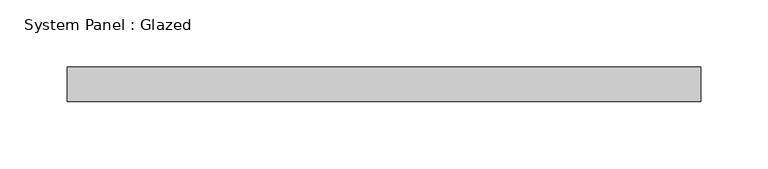
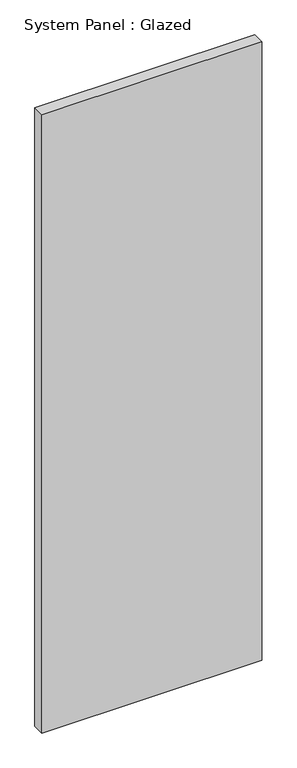
"""IFC4 building model written with IfcOpenShell, lengths in millimetres: plate geometry, System Panel : Glazed."""

from ifc_helpers import new_model, si_unit, origin, origin_with_axes, place, context, project, spatial, polyline, outline, extrude, source, transform, mapped, element, save


def system_panel_glazed_113fdc6f(model_context):
    return source(origin(), model_context, "Body", "SweptSolid", [
        extrude(outline(polyline([(234.95, 19.05), (-234.95, 19.05), (-234.95, 44.45), (234.95, 44.45), (234.95, 19.05)])), origin_with_axes(), (0.0, 0.0, 1.0), 1397.0),
    ])


if __name__ == "__main__":
    model = new_model("IFC4")
    model_context = context("Model", 3, world=origin())
    ifc_project = project(units=[si_unit("LENGTHUNIT", "METRE", prefix="MILLI")], contexts=[model_context])
    site = spatial("IfcSite", under=ifc_project)
    building = spatial("IfcBuilding", under=site)
    placement = place(None, origin())
    system_panel_glazed_shape = system_panel_glazed_113fdc6f(model_context)
    element("IfcPlate", 1, ObjectType="System Panel : Glazed", at=placement, inside=building, context=model_context, shape_type="MappedRepresentation", body=[
        mapped(system_panel_glazed_shape, transform((0.0, 0.0, 0.0), x_axis=(1.0, 0.0, 0.0), y_axis=(0.0, 1.0, 0.0), z_axis=(0.0, 0.0, 1.0))),
    ])
    save(model, "model.ifc")

# Revit data of these elements
# Type "System Panel : Glazed"
#   Construction Type Id = "GSP4R"
#   Analytic Construction = "1/8 in Pilkington single glazing"
#   Visual Light Transmittance = 0.9
#   Solar Heat Gain Coefficient = 0.86
#   Heat Transfer Coefficient (U) = 1.18115 BTU/(h·ft²·°F)
#   Define Thermal Properties by = 1
# Element 1 (IfcPlate, "System Panel : Glazed")
#   Materials on its faces: "Glass"
# Materials
#   "Glass": class "Glass", colour RGB 0 128 192, transparency 0.75, Description = "Soda Lime Glass", Cost = 0
